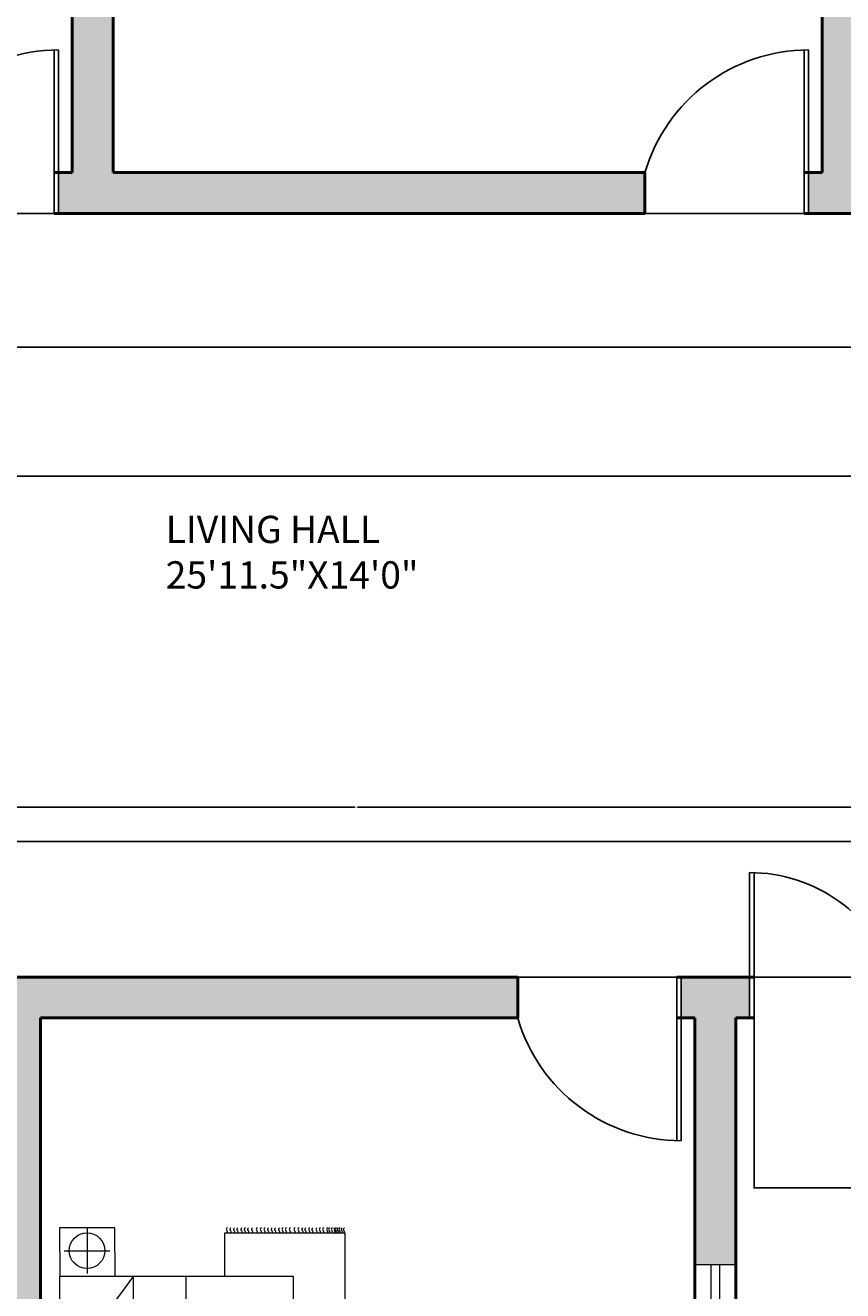
# Model space of a CAD drawing. Units: inches. Extents: x 383 to 970, y 275 to 1088.
# Tile 6 of 11: x 579 to 759, y 546 to 825. Entities that reach past the tile are written whole.
import ezdxf

# ---------------------------------------------------------------- set-up
doc = ezdxf.new("R2010")
doc.units = ezdxf.units.IN
doc.header["$MEASUREMENT"] = 0
for name, color, linetype, lineweight in [('A-ANNO-DIMS', 2, 'Continuous', 18), ('A-AREA-IDEN', 7, 'Continuous', 18), ('A-DOOR', 3, 'Continuous', 25), ('A-FURN', 8, 'Continuous', 18), ('A-GLAZ', 4, 'Continuous', 18), ('A-WALL', 7, 'Continuous', 50)]:
    doc.layers.add(name, color=color, linetype=linetype, lineweight=lineweight)
doc.layers.add('A-WALL-PATT', color=251, linetype='Continuous', lineweight=13, true_color=0x636466)
doc.styles.get("Standard").update_dxf_attribs({"font": 'arial.ttf'})
doc.dimstyles.get("Standard").update_dxf_attribs({"dimtxt": 0.18, "dimasz": 0.18, "dimexe": 0.18, "dimexo": 0.0625, "dimgap": 0.09, "dimtad": 0, "dimtih": 1, "dimtoh": 1, "dimdec": 4, "dimzin": 0, "dimdsep": 46, "dimtxsty": 'Standard', "dimcen": 0.09, "dimadec": 0, "dimazin": 0, "dimtfac": 1, "dimtdec": 4, "dimtofl": 0, "dimtmove": 0, "dimatfit": 3, "dimfxl": 1, "dimtolj": 1, "dimtzin": 0, "dimarcsym": 0})

# ---------------------------------------------------------------- blocks, each defined once
blk = doc.blocks.new('BED-DOUBLE-WITH-NIGHTSTANDS')
for p, q in [((6.09, 68.68), (6.09, 58.62)), ((36.42, 67.59), (62.78, 67.59)), ((36.42, 58.05), (36.42, 67.59)), ((62.78, 67.59), (62.78, 4.35)), ((1.07, 63.65), (11.12, 63.65)), ((9.97, 49.39), (16.32, 58)), ((16.32, 49.44), (16.32, 58)), ((27.82, 58.05), (27.82, 10.63)), ((9.97, 49.44), (16.32, 49.44)), ((9.97, 49.39), (9.97, 10.63)), ((10.78, 49.44), (10.78, 10.63)), ((6.2, 10.63), (6.2, 0.57)), ((36.42, 4.35), (36.42, 10.65)), ((1.17, 5.6), (11.22, 5.6)), ((62.78, 4.35), (36.42, 4.35))]:
    blk.add_line(p, q)
for points in [[(12.29, 58.05), (12.19, 68.68), (0, 68.68), (0.1, 58.05)], [(0.1, 58.05), (51.42, 58.05), (51.42, 10.63), (0.1, 10.63)], [(2.8, 49.44), (9.97, 49.44), (9.97, 35.55), (2.8, 35.55)], [(2.8, 29.88), (9.97, 29.88), (9.97, 15.98), (2.8, 15.98)], [(12.39, 0), (12.29, 10.63), (0.1, 10.63), (0.21, 0)]]:
    blk.add_lwpolyline(points, close=True)
for centre in [(6.09, 63.65), (6.2, 5.6)]:
    blk.add_circle(centre, 3.92)
for points, knots in [([(36.95, 68.71), (36.83, 68.61), (36.59, 68.42), (36.83, 68.08), (37, 67.8), (36.89, 67.65), (36.85, 67.58)], [0, 0, 0, 0, 0.400747, 0.791423, 1.067667, 1.29709, 1.29709, 1.29709, 1.29709]), ([(37.73, 68.71), (37.61, 68.61), (37.37, 68.42), (37.61, 68.08), (37.78, 67.8), (37.67, 67.65), (37.62, 67.58)], [0, 0, 0, 0, 0.400747, 0.791423, 1.067667, 1.29709, 1.29709, 1.29709, 1.29709]), ([(38.54, 68.71), (38.42, 68.61), (38.18, 68.42), (38.42, 68.08), (38.59, 67.8), (38.49, 67.65), (38.44, 67.58)], [0, 0, 0, 0, 0.400747, 0.791423, 1.067667, 1.29709, 1.29709, 1.29709, 1.29709]), ([(39.27, 68.71), (39.15, 68.61), (38.91, 68.42), (39.15, 68.08), (39.32, 67.8), (39.22, 67.65), (39.17, 67.58)], [0, 0, 0, 0, 0.400747, 0.791423, 1.067667, 1.29709, 1.29709, 1.29709, 1.29709]), ([(40.15, 68.71), (40.03, 68.61), (39.79, 68.42), (40.03, 68.08), (40.21, 67.8), (40.1, 67.65), (40.05, 67.58)], [0, 0, 0, 0, 0.400747, 0.791423, 1.067667, 1.29709, 1.29709, 1.29709, 1.29709]), ([(40.91, 68.71), (40.78, 68.61), (40.54, 68.42), (40.78, 68.08), (40.96, 67.8), (40.85, 67.65), (40.8, 67.58)], [0, 0, 0, 0, 0.400747, 0.791423, 1.067667, 1.29709, 1.29709, 1.29709, 1.29709]), ([(41.63, 68.71), (41.51, 68.61), (41.27, 68.42), (41.51, 68.08), (41.69, 67.8), (41.58, 67.65), (41.53, 67.58)], [0, 0, 0, 0, 0.400747, 0.791423, 1.067667, 1.29709, 1.29709, 1.29709, 1.29709]), ([(42.52, 68.71), (42.39, 68.61), (42.16, 68.42), (42.39, 68.08), (42.57, 67.8), (42.46, 67.65), (42.41, 67.58)], [0, 0, 0, 0, 0.400747, 0.791423, 1.067667, 1.29709, 1.29709, 1.29709, 1.29709]), ([(43.55, 68.71), (43.43, 68.61), (43.19, 68.42), (43.43, 68.08), (43.6, 67.8), (43.5, 67.65), (43.45, 67.58)], [0, 0, 0, 0, 0.400747, 0.791423, 1.067667, 1.29709, 1.29709, 1.29709, 1.29709]), ([(44.43, 68.71), (44.31, 68.61), (44.07, 68.42), (44.31, 68.08), (44.49, 67.8), (44.38, 67.65), (44.33, 67.58)], [0, 0, 0, 0, 0.400747, 0.791423, 1.067667, 1.29709, 1.29709, 1.29709, 1.29709]), ([(45.25, 68.71), (45.13, 68.61), (44.89, 68.42), (45.13, 68.08), (45.3, 67.8), (45.2, 67.65), (45.15, 67.58)], [0, 0, 0, 0, 0.400747, 0.791423, 1.067667, 1.29709, 1.29709, 1.29709, 1.29709]), ([(46.03, 68.71), (45.91, 68.61), (45.67, 68.42), (45.91, 68.08), (46.08, 67.8), (45.97, 67.65), (45.92, 67.58)], [0, 0, 0, 0, 0.400747, 0.791423, 1.067667, 1.29709, 1.29709, 1.29709, 1.29709]), ([(46.84, 68.71), (46.72, 68.61), (46.48, 68.42), (46.72, 68.08), (46.9, 67.8), (46.79, 67.65), (46.74, 67.58)], [0, 0, 0, 0, 0.400747, 0.791423, 1.067667, 1.29709, 1.29709, 1.29709, 1.29709]), ([(47.57, 68.71), (47.45, 68.61), (47.21, 68.42), (47.45, 68.08), (47.62, 67.8), (47.52, 67.65), (47.47, 67.58)], [0, 0, 0, 0, 0.400747, 0.791423, 1.067667, 1.29709, 1.29709, 1.29709, 1.29709]), ([(48.45, 68.71), (48.33, 68.61), (48.09, 68.42), (48.33, 68.08), (48.51, 67.8), (48.4, 67.65), (48.35, 67.58)], [0, 0, 0, 0, 0.400747, 0.791423, 1.067667, 1.29709, 1.29709, 1.29709, 1.29709]), ([(49.21, 68.71), (49.08, 68.61), (48.85, 68.42), (49.08, 68.08), (49.26, 67.8), (49.15, 67.65), (49.1, 67.58)], [0, 0, 0, 0, 0.400747, 0.791423, 1.067667, 1.29709, 1.29709, 1.29709, 1.29709]), ([(49.93, 68.71), (49.81, 68.61), (49.57, 68.42), (49.81, 68.08), (49.99, 67.8), (49.88, 67.65), (49.83, 67.58)], [0, 0, 0, 0, 0.400747, 0.791423, 1.067667, 1.29709, 1.29709, 1.29709, 1.29709]), ([(50.82, 68.71), (50.69, 68.61), (50.46, 68.42), (50.69, 68.08), (50.87, 67.8), (50.76, 67.65), (50.71, 67.58)], [0, 0, 0, 0, 0.400747, 0.791423, 1.067667, 1.29709, 1.29709, 1.29709, 1.29709]), ([(51.85, 68.71), (51.73, 68.61), (51.49, 68.42), (51.73, 68.08), (51.9, 67.8), (51.8, 67.65), (51.75, 67.58)], [0, 0, 0, 0, 0.400747, 0.791423, 1.067667, 1.29709, 1.29709, 1.29709, 1.29709]), ([(52.74, 68.71), (52.61, 68.61), (52.37, 68.42), (52.61, 68.08), (52.79, 67.8), (52.68, 67.65), (52.63, 67.58)], [0, 0, 0, 0, 0.400747, 0.791423, 1.067667, 1.29709, 1.29709, 1.29709, 1.29709]), ([(53.55, 68.71), (53.43, 68.61), (53.19, 68.42), (53.43, 68.08), (53.6, 67.8), (53.5, 67.65), (53.45, 67.58)], [0, 0, 0, 0, 0.400747, 0.791423, 1.067667, 1.29709, 1.29709, 1.29709, 1.29709]), ([(54.24, 68.71), (54.12, 68.61), (53.88, 68.42), (54.12, 68.08), (54.29, 67.8), (54.19, 67.65), (54.14, 67.58)], [0, 0, 0, 0, 0.400747, 0.791423, 1.067667, 1.29709, 1.29709, 1.29709, 1.29709]), ([(55.06, 68.71), (54.94, 68.61), (54.7, 68.42), (54.94, 68.08), (55.11, 67.8), (55, 67.65), (54.95, 67.58)], [0, 0, 0, 0, 0.400747, 0.791423, 1.067667, 1.29709, 1.29709, 1.29709, 1.29709]), ([(55.78, 68.71), (55.66, 68.61), (55.42, 68.42), (55.66, 68.08), (55.84, 67.8), (55.73, 67.65), (55.68, 67.58)], [0, 0, 0, 0, 0.400747, 0.791423, 1.067667, 1.29709, 1.29709, 1.29709, 1.29709]), ([(56.67, 68.71), (56.55, 68.61), (56.31, 68.42), (56.55, 68.08), (56.72, 67.8), (56.61, 67.65), (56.56, 67.58)], [0, 0, 0, 0, 0.400747, 0.791423, 1.067667, 1.29709, 1.29709, 1.29709, 1.29709]), ([(57.42, 68.71), (57.3, 68.61), (57.06, 68.42), (57.3, 68.08), (57.47, 67.8), (57.36, 67.65), (57.32, 67.58)], [0, 0, 0, 0, 0.400747, 0.791423, 1.067667, 1.29709, 1.29709, 1.29709, 1.29709]), ([(58.15, 68.71), (58.03, 68.61), (57.79, 68.42), (58.03, 68.08), (58.2, 67.8), (58.1, 67.66), (58.05, 67.59)], [0, 0, 0, 0, 0.400747, 0.791423, 1.067667, 1.283686, 1.283686, 1.283686, 1.283686]), ([(59.03, 68.71), (58.91, 68.61), (58.67, 68.42), (58.91, 68.08), (59.08, 67.8), (58.98, 67.66), (58.93, 67.59)], [0, 0, 0, 0, 0.400747, 0.791423, 1.067667, 1.283686, 1.283686, 1.283686, 1.283686]), ([(59.46, 68.71), (59.34, 68.61), (59.09, 68.42), (59.34, 68.08), (59.51, 67.8), (59.41, 67.66), (59.36, 67.59)], [0, 0, 0, 0, 0.402903, 0.794912, 1.071156, 1.287177, 1.287177, 1.287177, 1.287177]), ([(60.05, 68.71), (59.93, 68.61), (59.69, 68.42), (59.93, 68.08), (60.1, 67.8), (60, 67.66), (59.96, 67.59)], [0, 0, 0, 0, 0.400747, 0.791423, 1.067667, 1.283686, 1.283686, 1.283686, 1.283686]), ([(60.63, 68.71), (60.51, 68.61), (60.27, 68.42), (60.51, 68.08), (60.68, 67.8), (60.58, 67.66), (60.53, 67.59)], [0, 0, 0, 0, 0.400747, 0.791423, 1.067667, 1.283686, 1.283686, 1.283686, 1.283686]), ([(60.94, 68.71), (60.82, 68.61), (60.58, 68.42), (60.81, 68.08), (60.99, 67.8), (60.89, 67.66), (60.84, 67.59)], [0, 0, 0, 0, 0.400747, 0.791423, 1.067667, 1.283686, 1.283686, 1.283686, 1.283686]), ([(61.36, 68.71), (61.23, 68.61), (60.99, 68.42), (61.23, 68.08), (61.41, 67.8), (61.3, 67.65), (61.25, 67.58)], [0, 0, 0, 0, 0.400747, 0.791423, 1.067667, 1.29709, 1.29709, 1.29709, 1.29709]), ([(61.75, 68.71), (61.63, 68.61), (61.39, 68.42), (61.63, 68.08), (61.8, 67.8), (61.7, 67.65), (61.65, 67.58)], [0, 0, 0, 0, 0.400747, 0.791423, 1.067667, 1.29709, 1.29709, 1.29709, 1.29709]), ([(62.24, 68.71), (62.12, 68.61), (61.88, 68.42), (62.12, 68.08), (62.29, 67.8), (62.18, 67.65), (62.13, 67.58)], [0, 0, 0, 0, 0.400747, 0.791423, 1.067667, 1.29709, 1.29709, 1.29709, 1.29709]), ([(62.71, 68.71), (62.59, 68.61), (62.35, 68.42), (62.59, 68.08), (62.76, 67.8), (62.66, 67.65), (62.61, 67.58)], [0, 0, 0, 0, 0.400747, 0.791423, 1.067667, 1.29709, 1.29709, 1.29709, 1.29709]), ([(36.95, 3.23), (36.83, 3.32), (36.59, 3.52), (36.83, 3.86), (37, 4.14), (36.89, 4.29), (36.85, 4.35)], [0, 0, 0, 0, 0.400747, 0.791423, 1.067667, 1.29709, 1.29709, 1.29709, 1.29709]), ([(37.73, 3.23), (37.61, 3.32), (37.37, 3.52), (37.61, 3.86), (37.78, 4.14), (37.67, 4.29), (37.62, 4.35)], [0, 0, 0, 0, 0.400747, 0.791423, 1.067667, 1.29709, 1.29709, 1.29709, 1.29709]), ([(38.54, 3.23), (38.42, 3.32), (38.18, 3.52), (38.42, 3.86), (38.59, 4.14), (38.49, 4.29), (38.44, 4.35)], [0, 0, 0, 0, 0.400747, 0.791423, 1.067667, 1.29709, 1.29709, 1.29709, 1.29709]), ([(39.27, 3.23), (39.15, 3.32), (38.91, 3.52), (39.15, 3.86), (39.32, 4.14), (39.22, 4.29), (39.17, 4.35)], [0, 0, 0, 0, 0.400747, 0.791423, 1.067667, 1.29709, 1.29709, 1.29709, 1.29709]), ([(40.15, 3.23), (40.03, 3.32), (39.79, 3.52), (40.03, 3.86), (40.21, 4.14), (40.1, 4.29), (40.05, 4.35)], [0, 0, 0, 0, 0.400747, 0.791423, 1.067667, 1.29709, 1.29709, 1.29709, 1.29709]), ([(40.91, 3.23), (40.78, 3.32), (40.54, 3.52), (40.78, 3.86), (40.96, 4.14), (40.85, 4.29), (40.8, 4.35)], [0, 0, 0, 0, 0.400747, 0.791423, 1.067667, 1.29709, 1.29709, 1.29709, 1.29709]), ([(41.63, 3.23), (41.51, 3.32), (41.27, 3.52), (41.51, 3.86), (41.69, 4.14), (41.58, 4.29), (41.53, 4.35)], [0, 0, 0, 0, 0.400747, 0.791423, 1.067667, 1.29709, 1.29709, 1.29709, 1.29709]), ([(42.52, 3.23), (42.39, 3.32), (42.16, 3.52), (42.39, 3.86), (42.57, 4.14), (42.46, 4.29), (42.41, 4.35)], [0, 0, 0, 0, 0.400747, 0.791423, 1.067667, 1.29709, 1.29709, 1.29709, 1.29709]), ([(43.55, 3.23), (43.43, 3.32), (43.19, 3.52), (43.43, 3.86), (43.6, 4.14), (43.5, 4.29), (43.45, 4.35)], [0, 0, 0, 0, 0.400747, 0.791423, 1.067667, 1.29709, 1.29709, 1.29709, 1.29709]), ([(44.43, 3.23), (44.31, 3.32), (44.07, 3.52), (44.31, 3.86), (44.49, 4.14), (44.38, 4.29), (44.33, 4.35)], [0, 0, 0, 0, 0.400747, 0.791423, 1.067667, 1.29709, 1.29709, 1.29709, 1.29709]), ([(45.25, 3.23), (45.13, 3.32), (44.89, 3.52), (45.13, 3.86), (45.3, 4.14), (45.2, 4.29), (45.15, 4.35)], [0, 0, 0, 0, 0.400747, 0.791423, 1.067667, 1.29709, 1.29709, 1.29709, 1.29709]), ([(46.03, 3.23), (45.91, 3.32), (45.67, 3.52), (45.91, 3.86), (46.08, 4.14), (45.97, 4.29), (45.92, 4.35)], [0, 0, 0, 0, 0.400747, 0.791423, 1.067667, 1.29709, 1.29709, 1.29709, 1.29709]), ([(46.84, 3.23), (46.72, 3.32), (46.48, 3.52), (46.72, 3.86), (46.9, 4.14), (46.79, 4.29), (46.74, 4.35)], [0, 0, 0, 0, 0.400747, 0.791423, 1.067667, 1.29709, 1.29709, 1.29709, 1.29709]), ([(47.57, 3.23), (47.45, 3.32), (47.21, 3.52), (47.45, 3.86), (47.62, 4.14), (47.52, 4.29), (47.47, 4.35)], [0, 0, 0, 0, 0.400747, 0.791423, 1.067667, 1.29709, 1.29709, 1.29709, 1.29709]), ([(48.45, 3.23), (48.33, 3.32), (48.09, 3.52), (48.33, 3.86), (48.51, 4.14), (48.4, 4.29), (48.35, 4.35)], [0, 0, 0, 0, 0.400747, 0.791423, 1.067667, 1.29709, 1.29709, 1.29709, 1.29709]), ([(49.21, 3.23), (49.08, 3.32), (48.85, 3.52), (49.08, 3.86), (49.26, 4.14), (49.15, 4.29), (49.1, 4.35)], [0, 0, 0, 0, 0.400747, 0.791423, 1.067667, 1.29709, 1.29709, 1.29709, 1.29709]), ([(49.93, 3.23), (49.81, 3.32), (49.57, 3.52), (49.81, 3.86), (49.99, 4.14), (49.88, 4.29), (49.83, 4.35)], [0, 0, 0, 0, 0.400747, 0.791423, 1.067667, 1.29709, 1.29709, 1.29709, 1.29709]), ([(50.82, 3.23), (50.69, 3.32), (50.46, 3.52), (50.69, 3.86), (50.87, 4.14), (50.76, 4.29), (50.71, 4.35)], [0, 0, 0, 0, 0.400747, 0.791423, 1.067667, 1.29709, 1.29709, 1.29709, 1.29709]), ([(51.85, 3.23), (51.73, 3.32), (51.49, 3.52), (51.73, 3.86), (51.9, 4.14), (51.8, 4.29), (51.75, 4.35)], [0, 0, 0, 0, 0.400747, 0.791423, 1.067667, 1.29709, 1.29709, 1.29709, 1.29709]), ([(52.74, 3.23), (52.61, 3.32), (52.37, 3.52), (52.61, 3.86), (52.79, 4.14), (52.68, 4.29), (52.63, 4.35)], [0, 0, 0, 0, 0.400747, 0.791423, 1.067667, 1.29709, 1.29709, 1.29709, 1.29709]), ([(53.55, 3.23), (53.43, 3.32), (53.19, 3.52), (53.43, 3.86), (53.6, 4.14), (53.5, 4.29), (53.45, 4.35)], [0, 0, 0, 0, 0.400747, 0.791423, 1.067667, 1.29709, 1.29709, 1.29709, 1.29709]), ([(54.24, 3.23), (54.12, 3.32), (53.88, 3.52), (54.12, 3.86), (54.29, 4.14), (54.19, 4.29), (54.14, 4.35)], [0, 0, 0, 0, 0.400747, 0.791423, 1.067667, 1.29709, 1.29709, 1.29709, 1.29709]), ([(55.06, 3.23), (54.94, 3.32), (54.7, 3.52), (54.94, 3.86), (55.11, 4.14), (55, 4.29), (54.95, 4.35)], [0, 0, 0, 0, 0.400747, 0.791423, 1.067667, 1.29709, 1.29709, 1.29709, 1.29709]), ([(55.78, 3.23), (55.66, 3.32), (55.42, 3.52), (55.66, 3.86), (55.84, 4.14), (55.73, 4.29), (55.68, 4.35)], [0, 0, 0, 0, 0.400747, 0.791423, 1.067667, 1.29709, 1.29709, 1.29709, 1.29709]), ([(56.67, 3.23), (56.55, 3.32), (56.31, 3.52), (56.55, 3.86), (56.72, 4.14), (56.61, 4.29), (56.56, 4.35)], [0, 0, 0, 0, 0.400747, 0.791423, 1.067667, 1.29709, 1.29709, 1.29709, 1.29709]), ([(57.42, 3.23), (57.3, 3.32), (57.06, 3.52), (57.3, 3.86), (57.47, 4.14), (57.36, 4.29), (57.32, 4.35)], [0, 0, 0, 0, 0.400747, 0.791423, 1.067667, 1.29709, 1.29709, 1.29709, 1.29709]), ([(58.15, 3.23), (58.03, 3.32), (57.79, 3.52), (58.03, 3.86), (58.2, 4.14), (58.09, 4.29), (58.04, 4.35)], [0, 0, 0, 0, 0.400747, 0.791423, 1.067667, 1.29709, 1.29709, 1.29709, 1.29709]), ([(59.03, 3.23), (58.91, 3.32), (58.67, 3.52), (58.91, 3.86), (59.08, 4.14), (58.98, 4.29), (58.93, 4.35)], [0, 0, 0, 0, 0.400747, 0.791423, 1.067667, 1.29709, 1.29709, 1.29709, 1.29709]), ([(59.46, 3.23), (59.33, 3.32), (59.08, 3.52), (59.34, 3.86), (59.51, 4.14), (59.4, 4.29), (59.36, 4.35)], [0, 0, 0, 0, 0.407265, 0.802015, 1.07826, 1.307683, 1.307683, 1.307683, 1.307683]), ([(60.03, 3.23), (59.9, 3.32), (59.67, 3.52), (59.9, 3.86), (60.08, 4.14), (59.97, 4.29), (59.92, 4.35)], [0, 0, 0, 0, 0.400747, 0.791423, 1.067667, 1.29709, 1.29709, 1.29709, 1.29709]), ([(60.6, 3.23), (60.48, 3.32), (60.24, 3.52), (60.48, 3.86), (60.65, 4.14), (60.54, 4.29), (60.5, 4.35)], [0, 0, 0, 0, 0.400747, 0.791423, 1.067667, 1.29709, 1.29709, 1.29709, 1.29709]), ([(60.91, 3.23), (60.79, 3.32), (60.55, 3.52), (60.79, 3.86), (60.96, 4.14), (60.85, 4.29), (60.81, 4.35)], [0, 0, 0, 0, 0.400747, 0.791423, 1.067667, 1.29709, 1.29709, 1.29709, 1.29709]), ([(61.33, 3.23), (61.21, 3.32), (60.97, 3.52), (61.21, 3.86), (61.38, 4.14), (61.27, 4.29), (61.22, 4.35)], [0, 0, 0, 0, 0.400747, 0.791423, 1.067667, 1.29709, 1.29709, 1.29709, 1.29709]), ([(61.72, 3.23), (61.6, 3.32), (61.36, 3.52), (61.6, 3.86), (61.78, 4.14), (61.67, 4.29), (61.62, 4.35)], [0, 0, 0, 0, 0.400747, 0.791423, 1.067667, 1.29709, 1.29709, 1.29709, 1.29709]), ([(62.21, 3.23), (62.09, 3.32), (61.85, 3.52), (62.09, 3.86), (62.26, 4.14), (62.16, 4.29), (62.11, 4.35)], [0, 0, 0, 0, 0.400747, 0.791423, 1.067667, 1.29709, 1.29709, 1.29709, 1.29709]), ([(62.71, 3.23), (62.59, 3.32), (62.35, 3.52), (62.59, 3.86), (62.76, 4.14), (62.66, 4.29), (62.61, 4.35)], [0, 0, 0, 0, 0.400747, 0.791423, 1.067667, 1.29709, 1.29709, 1.29709, 1.29709])]:
    blk.add_open_spline(points, degree=3, knots=knots)
blk = doc.blocks.new('DOOR-LEAF-36IN')
for p, q in [((0, 0), (0, 36)), ((1, 36), (1, 0)), ((0, 0), (1, 0))]:
    blk.add_line(p, q)
blk.add_arc((0, -1.5), 37.5, 16.2602, 90)
blk = doc.blocks.new('WIN-60IN')
for p, q in [((60, 9), (0, 9)), ((60, 5.5), (0, 5.5)), ((0, 3.5), (60, 3.5)), ((0, 0), (60, 0))]:
    blk.add_line(p, q)
blk = doc.blocks.new('DOOR-LEAF-32IN')
for p, q in [((32, 32), (31, 32)), ((31, 0), (31, 32)), ((32, 32), (32, 0))]:
    blk.add_line(p, q)
blk.add_arc((32, 33.76), 33.76, 198.5866, 270)
blk = doc.blocks.new('*D53')
at = {"layer": 'A-ANNO-DIMS', "color": 0, "lineweight": -2, "transparency": 16777216}
for p, q in [((814.18, 783.14), (382.71, 783.14)), ((382.89, 782.96), (382.89, 768.63)), ((382.89, 753.94), (382.89, 768.27)), ((814.18, 753.76), (382.71, 753.76))]:
    blk.add_line(p, q, dxfattribs=at)
at = {"layer": 'A-ANNO-DIMS', "color": 0, "transparency": 16777216}
for points in [[(382.86, 782.96), (382.92, 782.96), (382.89, 783.14)], [(382.86, 753.94), (382.92, 753.94), (382.89, 753.76)]]:
    blk.add_solid(points, dxfattribs=at)
at = {"layer": 'Defpoints', "color": 0, "transparency": 16777216}
for p in [(814.24, 783.14), (382.89, 753.76), (814.24, 753.76)]:
    blk.add_point(p, dxfattribs=at)
at = {"layer": 'A-ANNO-DIMS', "color": 0, "transparency": 16777216, "insert": (382.89, 768.45), "char_height": 0.18, "attachment_point": 5}
blk.add_mtext('\\A1;29.38', dxfattribs=at)
blk = doc.blocks.new('*D54')
at = {"layer": 'A-ANNO-DIMS', "color": 0, "lineweight": -2, "transparency": 16777216}
for p, q in [((814.18, 644.96), (382.71, 644.96)), ((382.89, 644.78), (382.89, 630.23)), ((382.89, 615.32), (382.89, 629.86)), ((814.18, 615.14), (382.71, 615.14))]:
    blk.add_line(p, q, dxfattribs=at)
at = {"layer": 'A-ANNO-DIMS', "color": 0, "transparency": 16777216}
for points in [[(382.86, 644.78), (382.92, 644.78), (382.89, 644.96)], [(382.86, 615.32), (382.92, 615.32), (382.89, 615.14)]]:
    blk.add_solid(points, dxfattribs=at)
at = {"layer": 'Defpoints', "color": 0, "transparency": 16777216}
for p in [(382.89, 644.96), (814.24, 644.96), (814.24, 615.14)]:
    blk.add_point(p, dxfattribs=at)
at = {"layer": 'A-ANNO-DIMS', "color": 0, "transparency": 16777216, "insert": (382.89, 630.05), "char_height": 0.18, "attachment_point": 5}
blk.add_mtext('\\A1;29.82', dxfattribs=at)
blk = doc.blocks.new('*D56')
at = {"layer": 'A-ANNO-DIMS', "color": 0, "lineweight": -2, "transparency": 16777216}
for p, q in [((805.18, 783.14), (382.71, 783.14)), ((382.89, 782.96), (382.89, 754.44)), ((382.89, 725.56), (382.89, 754.08)), ((805.18, 725.38), (382.71, 725.38))]:
    blk.add_line(p, q, dxfattribs=at)
at = {"layer": 'A-ANNO-DIMS', "color": 0, "transparency": 16777216}
for points in [[(382.86, 782.96), (382.92, 782.96), (382.89, 783.14)], [(382.86, 725.56), (382.92, 725.56), (382.89, 725.38)]]:
    blk.add_solid(points, dxfattribs=at)
at = {"layer": 'Defpoints', "color": 0, "transparency": 16777216}
for p in [(382.89, 783.14), (805.24, 783.14), (805.24, 725.38)]:
    blk.add_point(p, dxfattribs=at)
at = {"layer": 'A-ANNO-DIMS', "color": 0, "transparency": 16777216, "insert": (382.89, 754.26), "char_height": 0.18, "attachment_point": 5}
blk.add_mtext('\\A1;57.76', dxfattribs=at)
blk = doc.blocks.new('*D67')
at = {"layer": 'A-ANNO-DIMS', "color": 0, "lineweight": -2, "transparency": 16777216}
for p, q in [((498.24, 615.2), (498.24, 652.67)), ((498.42, 652.49), (651.45, 652.49)), ((805.06, 652.49), (652.03, 652.49)), ((805.24, 615.2), (805.24, 652.67))]:
    blk.add_line(p, q, dxfattribs=at)
at = {"layer": 'A-ANNO-DIMS', "color": 0, "transparency": 16777216}
for points in [[(498.42, 652.52), (498.42, 652.46), (498.24, 652.49)], [(805.06, 652.52), (805.06, 652.46), (805.24, 652.49)]]:
    blk.add_solid(points, dxfattribs=at)
at = {"layer": 'Defpoints', "color": 0, "transparency": 16777216}
for p in [(805.24, 652.49), (498.24, 615.14), (805.24, 615.14)]:
    blk.add_point(p, dxfattribs=at)
at = {"layer": 'A-ANNO-DIMS', "color": 0, "transparency": 16777216, "insert": (651.74, 652.49), "char_height": 0.18, "attachment_point": 5}
blk.add_mtext('\\A1;307', dxfattribs=at)
blk = doc.blocks.new('*D68')
at = {"layer": 'A-ANNO-DIMS', "color": 0, "lineweight": -2, "transparency": 16777216}
for p, q in [((739.24, 606.07), (739.24, 568.61)), ((801.24, 606.07), (801.24, 568.61)), ((739.42, 568.79), (770.02, 568.79)), ((801.06, 568.79), (770.46, 568.79))]:
    blk.add_line(p, q, dxfattribs=at)
at = {"layer": 'A-ANNO-DIMS', "color": 0, "transparency": 16777216}
for points in [[(739.42, 568.82), (739.42, 568.76), (739.24, 568.79)], [(801.06, 568.82), (801.06, 568.76), (801.24, 568.79)]]:
    blk.add_solid(points, dxfattribs=at)
at = {"layer": 'Defpoints', "color": 0, "transparency": 16777216}
for p in [(739.24, 606.14), (801.24, 606.14), (739.24, 568.79)]:
    blk.add_point(p, dxfattribs=at)
at = {"layer": 'A-ANNO-DIMS', "color": 0, "transparency": 16777216, "insert": (770.24, 568.79), "char_height": 0.18, "attachment_point": 5}
blk.add_mtext('\\A1;62', dxfattribs=at)

msp = doc.modelspace()

# ---------------------------------------------------------------- hatches: boundary and pattern name
at = {"layer": 'A-WALL-PATT'}
h = msp.add_hatch(color=256, dxfattribs=at)
h.dxf.hatch_style = 1
h.paths.add_polyline_path([(651.24, 321.1365), (651.24, 417.1365), (735.24, 417.1365), (735.24, 491.9233), (726.24, 491.9233), (726.24, 426.1365), (582.24, 426.1365), (582.24, 606.1365), (687.24, 606.1365), (687.24, 615.1365), (573.24, 615.1365), (573.24, 546.1365), (570.24, 546.1365), (570.24, 537.1365), (573.24, 537.1365), (573.24, 414.1365), (582.24, 414.1365), (582.24, 417.1365), (642.24, 417.1365), (642.24, 321.1365), (621.6203, 321.1365), (621.6203, 312.1365), (651.24, 312.1365)], flags=17)
h.paths.add_polyline_path([(597.6203, 321.1365), (582.24, 321.1365), (582.24, 390.1365), (573.24, 390.1365), (573.24, 321.1365), (570.24, 321.1365), (570.24, 312.1365), (573.24, 312.1365), (597.6203, 312.1365)], flags=16)
h.paths.add_polyline_path([(534.24, 321.1365), (500.8868, 321.1365), (500.8868, 312.1365), (534.24, 312.1365)], flags=17)
h.paths.add_polyline_path([(735.24, 606.1365), (738.24, 606.1365), (738.24, 615.1365), (723.24, 615.1365), (723.24, 606.1365), (726.24, 606.1365), (726.24, 551.9233), (735.24, 551.9233)], flags=17)
h.paths.add_polyline_path([(848.0899, 615.1365), (814.24, 615.1365), (814.24, 689.38), (805.24, 689.38), (805.24, 615.1365), (802.24, 615.1365), (802.24, 606.1365), (848.0899, 606.1365)], flags=17)
h.paths.add_polyline_path([(530.24, 615.1365), (498.24, 615.1365), (498.24, 646.5351), (489.24, 646.5351), (489.24, 615.1365), (466.771, 615.1365), (466.771, 606.1365), (521.24, 606.1365), (521.24, 603.1365), (530.24, 603.1365), (530.24, 606.1365)], flags=17)
h.paths.add_polyline_path([(498.24, 744.1365), (489.24, 744.1365), (489.24, 706.5351), (498.24, 706.5351)], flags=17)
h.paths.add_polyline_path([(715.24, 792.1365), (598.24, 792.1365), (598.24, 972.1365), (636.5058, 972.1365), (636.5058, 981.1365), (589.24, 981.1365), (589.24, 972.1365), (589.24, 792.1365), (586.24, 792.1365), (586.24, 783.1365), (589.24, 783.1365), (715.24, 783.1365)], flags=17)
h.paths.add_polyline_path([(763.24, 981.1365), (696.5058, 981.1365), (696.5058, 972.1365), (754.24, 972.1365), (754.24, 792.1365), (751.24, 792.1365), (751.24, 783.1365), (754.24, 783.1365), (764.24, 783.1365), (764.24, 792.1365), (763.24, 792.1365)], flags=17)
h.paths.add_polyline_path([(815.24, 1001.9492), (806.24, 1001.9492), (806.24, 972.1365), (818.24, 972.1365), (818.24, 981.1365), (815.24, 981.1365)], flags=17)
h.paths.add_polyline_path([(546.24, 1004.0336), (537.24, 1004.0336), (537.24, 981.1365), (534.24, 981.1365), (534.24, 972.1365), (537.24, 972.1365), (546.24, 972.1365), (546.24, 981.1365)], flags=17)
h.paths.add_polyline_path([(884.0899, 606.1365), (932.24, 606.1365), (932.24, 1050.1365), (420.24, 1050.1365), (420.24, 312.1365), (440.8868, 312.1365), (440.8868, 321.1365), (429.24, 321.1365), (429.24, 537.1365), (538.24, 537.1365), (538.24, 546.1365), (530.24, 546.1365), (530.24, 579.1365), (521.24, 579.1365), (521.24, 546.1365), (429.24, 546.1365), (429.24, 606.1365), (442.771, 606.1365), (442.771, 615.1365), (429.24, 615.1365), (429.24, 783.1365), (489.24, 783.1365), (489.24, 780.1365), (498.24, 780.1365), (498.24, 783.1365), (550.24, 783.1365), (550.24, 792.1365), (429.24, 792.1365), (429.24, 972.1365), (510.24, 972.1365), (510.24, 981.1365), (429.24, 981.1365), (429.24, 1041.1365), (537.24, 1041.1365), (537.24, 1028.0336), (546.24, 1028.0336), (546.24, 1041.1365), (806.24, 1041.1365), (806.24, 1025.9492), (815.24, 1025.9492), (815.24, 1041.1365), (923.24, 1041.1365), (923.24, 981.1365), (842.24, 981.1365), (842.24, 972.1365), (923.24, 972.1365), (923.24, 792.1365), (800.24, 792.1365), (800.24, 783.1365), (805.24, 783.1365), (805.24, 725.38), (814.24, 725.38), (814.24, 783.1365), (923.24, 783.1365), (923.24, 615.1365), (884.0899, 615.1365)])

# ---------------------------------------------------------------- linework, layer by layer
at = {"layer": 'A-DOOR'}
for p, q in [((586.24, 819.1365), (586.24, 783.1365)), ((751.24, 819.1365), (751.24, 783.1365)), ((738.24, 638.1365), (738.24, 606.1365)), ((723.24, 579.1365), (723.24, 615.1365))]:
    msp.add_line(p, q, dxfattribs=at)
at = {"layer": 'A-GLAZ'}
msp.add_line((726.24, 551.9233), (735.24, 551.9233), dxfattribs=at)
at = {"layer": 'A-WALL'}
for p, q in [((589.24, 981.1365), (589.24, 792.1365)), ((598.24, 972.1365), (598.24, 792.1365)), ((754.24, 972.1365), (754.24, 792.1365)), ((585.24, 792.1365), (589.24, 792.1365)), ((598.24, 792.1365), (715.24, 792.1365)), ((715.24, 783.1365), (715.24, 792.1365)), ((750.24, 792.1365), (754.24, 792.1365)), ((585.24, 783.1365), (715.24, 783.1365)), ((589.24, 783.1365), (586.24, 783.1365)), ((750.24, 783.1365), (765.24, 783.1365)), ((754.24, 783.1365), (751.24, 783.1365)), ((498.24, 615.1365), (687.24, 615.1365)), ((687.24, 615.1365), (687.24, 606.1365)), ((722.24, 615.1365), (739.24, 615.1365)), ((726.24, 615.1365), (723.24, 615.1365)), ((582.24, 606.1365), (582.24, 426.1365)), ((582.24, 606.1365), (687.24, 606.1365)), ((722.24, 606.1365), (726.24, 606.1365)), ((726.24, 606.1365), (726.24, 426.1365)), ((735.24, 606.1365), (735.24, 417.1365)), ((735.24, 606.1365), (738.24, 606.1365)), ((735.24, 606.1365), (739.24, 606.1365))]:
    msp.add_line(p, q, dxfattribs=at)

# ---------------------------------------------------------------- block references
at = {"layer": 'A-DOOR', "extrusion": (0, 0, -1), "zscale": -1}
for p in [(-586.2401, 783.136), (-751.2401, 783.136)]:
    msp.add_blockref('DOOR-LEAF-36IN', p, dxfattribs=at)
at = {"layer": 'A-DOOR', "rotation": 180}
for name, p in [('DOOR-LEAF-32IN', (770.2401, 638.137)), ('DOOR-LEAF-36IN', (723.2401, 615.137))]:
    msp.add_blockref(name, p, dxfattribs=at)
at = {"layer": 'A-FURN'}
msp.add_blockref('BED-DOUBLE-WITH-NIGHTSTANDS', (586.4226, 491.2789), dxfattribs=at)
at = {"layer": 'A-GLAZ', "rotation": 90.00000000000003}
msp.add_blockref('WIN-60IN', (735.2405, 491.9235), dxfattribs=at)

# ---------------------------------------------------------------- texts
at = {"layer": 'A-AREA-IDEN', "insert": (609.8156, 716.6302), "char_height": 6, "attachment_point": 1}
msp.add_mtext_dynamic_manual_height_columns('LIVING HALL\\P25\'11.5"X14\'0"', width=76.745999, gutter_width=30, heights=[0], dxfattribs=at)

# ---------------------------------------------------------------- dimensions: what is measured, and where the dimension line sits
at = {"layer": 'A-ANNO-DIMS'}
for base, p1, p2, angle, override, picture, middle in [((382.89, 753.7583), (814.24, 783.1365), (814.24, 753.7583), 90, {"dimdec": 2, "dimlfac": 1, "dimrnd": 0, "dimzin": 0, "dimdsep": 46, "dimlunit": 2}, '*D53', (382.89, 768.4474)), ((382.89, 783.1365), (805.24, 725.38), (805.24, 783.1365), 90, {"dimdec": 2, "dimlfac": 1, "dimrnd": 0, "dimzin": 0, "dimdsep": 46, "dimlunit": 2}, '*D56', (382.89, 754.2583)), ((382.89, 644.9565), (814.24, 615.1365), (814.24, 644.9565), 90, {"dimdec": 2, "dimlfac": 1, "dimrnd": 0, "dimzin": 0, "dimdsep": 46, "dimlunit": 2}, '*D54', (382.89, 630.0465)), ((739.24, 568.7865), (801.24, 606.1365), (739.24, 606.1365), 180, {"dimdec": 0, "dimlfac": 1, "dimrnd": 0, "dimzin": 0, "dimdsep": 46, "dimlunit": 2}, '*D68', (770.24, 568.7865))]:
    dim = msp.add_linear_dim(base=base, p1=p1, p2=p2, angle=angle, dimstyle='Standard', override=override, dxfattribs=at)
    dim.commit()
    dim.dimension.update_dxf_attribs({"geometry": picture, "text_midpoint": middle})
dim = msp.add_linear_dim(base=(805.24, 652.4865), p1=(498.24, 615.1365), p2=(805.24, 615.1365), dimstyle='Standard', override={"dimdec": 0, "dimlfac": 1, "dimrnd": 0, "dimzin": 0, "dimdsep": 46, "dimlunit": 2}, dxfattribs=at)
dim.commit()
dim.dimension.update_dxf_attribs({"geometry": '*D67', "text_midpoint": (651.74, 652.4865)})

doc.saveas('drawing.dxf')
